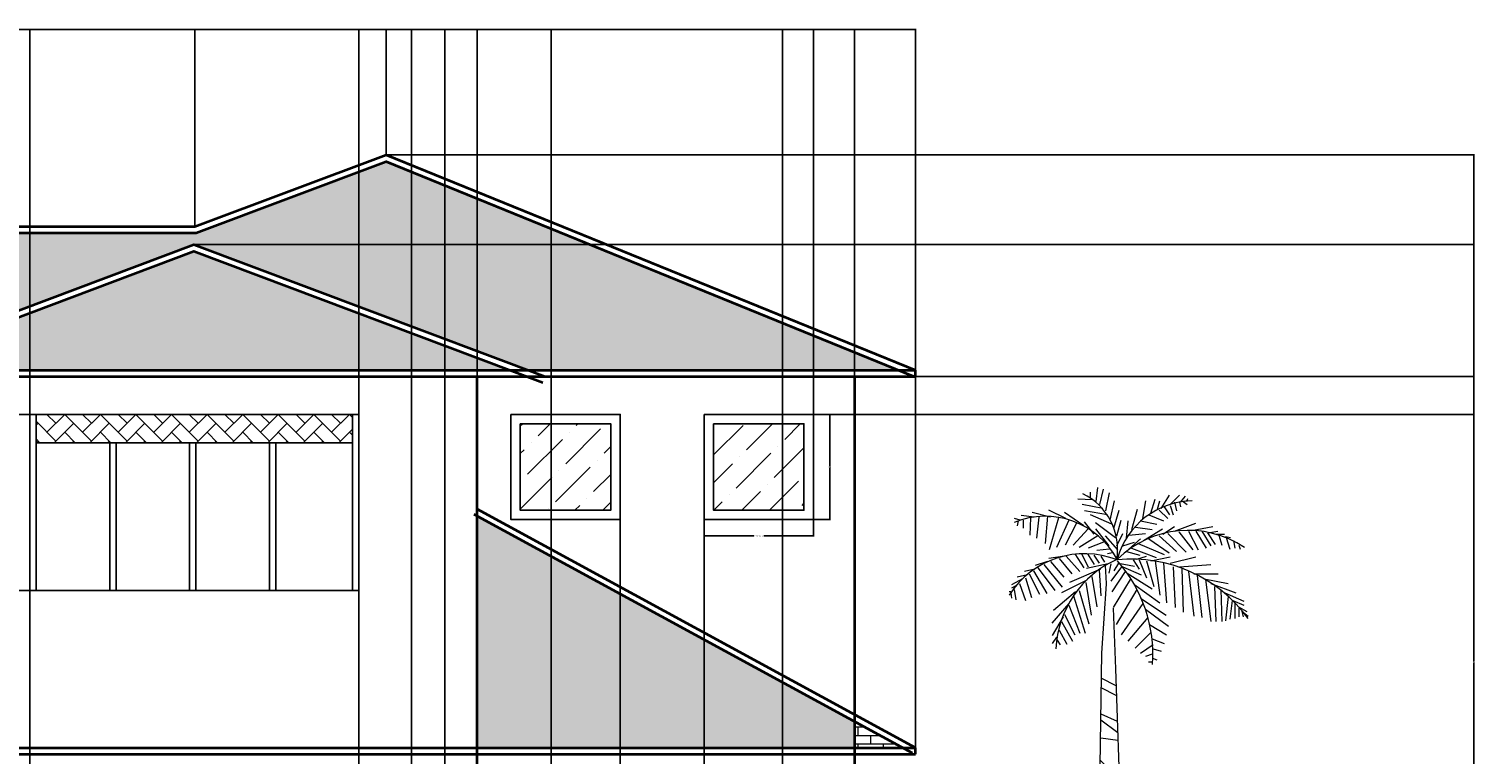
# Model space of a CAD drawing. Units: inches. Extents: x -177 to 697, y -125 to 346.
# Tile 4 of 4: x 237 to 697, y 116 to 346. Entities that reach past the tile are written whole.
import ezdxf

# ---------------------------------------------------------------- set-up
doc = ezdxf.new("R2010")
doc.units = ezdxf.units.IN
doc.header["$MEASUREMENT"] = 0
for name, color, linetype, lineweight in [('A-ANNO-DIMS', 2, 'Continuous', 18), ('A-GLAZ', 4, 'Continuous', 25), ('A-GLAZ-PATT', 252, 'Continuous', 13), ('A-ROOF', 1, 'Continuous', 35), ('A-ROOF-PATT', 252, 'Continuous', 13), ('A-WALL', 7, 'Continuous', 35), ('L-PLNT', 94, 'Continuous', 13)]:
    doc.layers.add(name, color=color, linetype=linetype, lineweight=lineweight)
doc.styles.get("Standard").update_dxf_attribs({"font": 'arial.ttf'})
doc.dimstyles.get("Standard").update_dxf_attribs({"dimtxt": 0.18, "dimasz": 0.18, "dimexe": 0.18, "dimexo": 0.0625, "dimgap": 0.09, "dimtad": 0, "dimtih": 1, "dimtoh": 1, "dimdec": 4, "dimzin": 0, "dimdsep": 46, "dimtxsty": 'Standard', "dimcen": 0.09, "dimadec": 0, "dimazin": 0, "dimtfac": 1, "dimtdec": 4, "dimtofl": 0, "dimtmove": 0, "dimatfit": 3, "dimfxl": 1, "dimtolj": 1, "dimtzin": 0, "dimarcsym": 0})
pattern_1 = [(0, (-118.8082, -115.7344), (0, 2.667), []), (90, (-118.808, -115.7344), (-4, 2.667), [2.667, -2.667])]

# ---------------------------------------------------------------- blocks, each defined once
blk = doc.blocks.new('*U2')
for p, q in [((-7.5, 199.68), (-7.5, 197.946)), ((-5.567, 196.707), (-4.987, 201.167)), ((-4.407, 195.716), (-3.247, 200.672)), ((-2.474, 193.733), (-1.315, 199.433)), ((15.116, 194.477), (17.822, 198.689)), ((18.015, 195.716), (20.914, 198.689)), ((21.301, 196.459), (22.847, 198.441)), ((-20.064, 191.751), (-25.863, 193.238)), ((-15.232, 191.255), (-20.644, 193.981)), ((-9.433, 189.025), (-15.618, 193.238)), ((-6.727, 197.202), (-11.366, 197.45)), ((-3.441, 194.477), (-10.013, 195.716)), ((-1.894, 192.494), (-9.24, 193.733)), ((-1.121, 190.759), (0.232, 196.955)), ((0.038, 188.281), (1.778, 193.981)), ((5.837, 187.786), (7.577, 194.229)), ((9.317, 191.255), (10.283, 196.955)), ((11.829, 192.99), (13.182, 197.45)), ((13.956, 194.229), (14.729, 196.955)), ((14.536, 193.981), (17.242, 191.255)), ((16.082, 194.972), (17.822, 192.494)), ((18.015, 195.468), (18.981, 192.494)), ((19.368, 196.459), (19.948, 193.733)), ((20.914, 196.459), (21.301, 194.972)), ((22.074, 196.707), (23.427, 195.716)), ((23.234, 196.707), (23.62, 197.698)), ((-29.729, 190.759), (-31.469, 191.255)), ((-30.309, 190.512), (-30.695, 189.025)), ((-25.283, 191.751), (-29.342, 192.246)), ((-28.763, 190.759), (-28.763, 188.281)), ((-26.443, 191.503), (-26.636, 186.051)), ((-23.737, 191.751), (-24.51, 185.06)), ((-21.031, 191.998), (-21.804, 183.325)), ((-17.551, 191.503), (-20.451, 181.343)), ((-14.265, 190.759), (-18.131, 182.086)), ((-11.753, 189.768), (-15.425, 182.83)), ((-6.147, 186.299), (-9.24, 190.264)), ((-0.541, 189.52), (-7.307, 192.494)), ((-5.76, 190.016), (0.618, 185.308)), ((1.005, 185.803), (2.358, 190.759)), ((4.098, 185.06), (4.678, 190.512)), ((8.544, 190.512), (13.763, 189.52)), ((11.25, 192.494), (15.889, 190.512)), ((15.695, 186.299), (19.368, 188.777)), ((19.368, 187.29), (26.133, 189.768)), ((24.78, 187.538), (31.546, 188.777)), ((-8.08, 188.034), (-12.912, 182.83)), ((-4.987, 185.803), (-10.979, 182.086)), ((-5.76, 188.034), (-1.508, 182.582)), ((-2.668, 185.803), (1.198, 181.343)), ((1.005, 182.582), (2.938, 186.547)), ((4.871, 186.051), (10.09, 186.547)), ((4.871, 181.591), (8.544, 184.812)), ((6.997, 188.529), (12.216, 187.786)), ((9.51, 184.317), (15.502, 188.034)), ((11.25, 184.812), (17.628, 180.352)), ((14.536, 185.803), (19.948, 180.847)), ((17.242, 186.547), (23.041, 180.599)), ((20.721, 187.042), (25.167, 181.343)), ((23.814, 187.29), (26.907, 181.343)), ((26.133, 187.29), (29.419, 181.838)), ((28.066, 187.29), (30.966, 182.582)), ((29.806, 186.795), (32.319, 183.078)), ((29.999, 186.795), (33.092, 187.29)), ((32.512, 186.299), (35.218, 186.299)), ((33.479, 186.051), (34.445, 182.83)), ((35.605, 185.556), (37.151, 185.308)), ((35.798, 185.308), (36.958, 181.591)), ((38.118, 184.317), (38.504, 181.838)), ((-15.618, 179.36), (-20.644, 178.617)), ((-15.038, 179.36), (-10.786, 174.404)), ((-12.332, 180.104), (-9.433, 175.643)), ((-10.206, 180.104), (-8.08, 175.891)), ((-8.273, 180.104), (-6.147, 176.635)), ((-3.247, 183.821), (-8.08, 181.838)), ((-6.34, 179.608), (-4.6, 177.13)), ((-1.315, 181.591), (-5.374, 181.095)), ((-4.021, 179.36), (-2.861, 177.378)), ((-0.348, 180.352), (-1.894, 180.104)), ((2.938, 182.582), (6.61, 183.821)), ((4.098, 180.847), (8.35, 179.608)), ((5.644, 181.838), (13.569, 178.865)), ((7.384, 178.369), (10.476, 179.36)), ((7.77, 183.325), (16.082, 179.856)), ((39.857, 182.83), (40.244, 181.591)), ((-25.09, 175.148), (-28.376, 174.404)), ((-21.031, 177.626), (-24.897, 176.387)), ((-24.317, 175.891), (-18.711, 168.457)), ((-22.191, 176.635), (-16.391, 169.448)), ((-20.064, 177.626), (-15.812, 172.67)), ((-17.358, 178.617), (-13.299, 173.661)), ((-4.214, 175.148), (-14.072, 170.935)), ((-1.701, 176.882), (-8.66, 175.396)), ((-4.6, 174.9), (-4.021, 166.722)), ((-2.668, 176.387), (-2.376, 170.594)), ((-0.928, 176.882), (-1.508, 173.909)), ((2.551, 175.891), (-0.928, 171.431)), ((1.585, 177.13), (0.038, 174.652)), ((1.585, 177.13), (6.61, 176.139)), ((2.938, 175.891), (8.737, 173.413)), ((6.224, 178.121), (8.157, 175.148)), ((8.157, 178.121), (10.476, 172.422)), ((10.476, 177.874), (12.796, 169.696)), ((11.829, 177.874), (18.015, 179.113)), ((13.182, 177.874), (14.729, 166.97)), ((15.889, 177.13), (16.855, 164.492)), ((18.015, 177.13), (26.133, 179.113)), ((18.981, 175.891), (19.561, 163.005)), ((20.914, 175.891), (30.966, 176.635)), ((21.688, 175.396), (22.074, 161.518)), ((-28.956, 172.174), (-32.435, 170.192)), ((-27.409, 173.413), (-30.695, 172.67)), ((-29.922, 170.687), (-27.989, 165.235)), ((-27.989, 172.422), (-26.056, 166.227)), ((-26.829, 173.661), (-23.544, 167.218)), ((-25.476, 174.652), (-21.224, 167.466)), ((-8.466, 171.678), (-16.585, 167.713)), ((-8.853, 170.935), (-7.113, 160.527)), ((-6.92, 172.917), (-5.374, 163.253)), ((3.711, 174.404), (-0.541, 167.961)), ((5.257, 171.926), (-0.155, 163.005)), ((4.291, 173.909), (12.216, 168.953)), ((6.417, 170.439), (14.729, 164.492)), ((23.814, 174.404), (25.554, 160.279)), ((25.554, 173.661), (33.285, 173.661)), ((26.52, 173.165), (28.066, 159.784)), ((28.839, 172.174), (36.378, 170.687)), ((29.226, 171.926), (30.966, 158.545)), ((30.966, 170.687), (38.891, 167.713)), ((-32.628, 167.961), (-33.208, 167.961)), ((-32.628, 167.713), (-32.435, 165.979)), ((-31.082, 169.944), (-32.435, 169.2)), ((-31.662, 168.705), (-31.082, 165.483)), ((-12.139, 167.961), (-19.098, 162.014)), ((-12.719, 166.722), (-9.046, 154.828)), ((-10.979, 168.457), (-7.887, 157.801)), ((7.384, 168.705), (0.812, 157.553)), ((8.544, 165.979), (16.662, 160.527)), ((32.126, 169.696), (32.512, 158.545)), ((34.058, 168.705), (34.445, 158.545)), ((35.412, 167.713), (41.404, 164.988)), ((36.378, 166.474), (35.605, 158.792)), ((-14.265, 164.244), (-19.678, 158.049)), ((-14.265, 163.749), (-10.786, 154.828)), ((9.317, 164.244), (2.358, 154.332)), ((10.09, 162.51), (17.435, 157.058)), ((37.731, 165.235), (36.958, 159.288)), ((37.924, 165.235), (41.404, 163.749)), ((38.504, 164.492), (38.504, 159.536)), ((39.664, 163.253), (42.37, 161.766)), ((39.857, 162.757), (39.857, 160.031)), ((40.824, 161.766), (41.21, 160.031)), ((41.21, 161.518), (42.757, 160.279)), ((-16.005, 160.031), (-19.484, 154.084)), ((-16.585, 158.545), (-13.106, 152.35)), ((-15.618, 160.775), (-12.332, 154.332)), ((10.863, 159.784), (4.484, 152.35)), ((11.443, 157.553), (16.855, 154.332)), ((-18.131, 153.589), (-19.484, 151.606)), ((-17.938, 152.597), (-16.972, 151.111)), ((-17.358, 155.819), (-14.845, 151.358)), ((11.829, 155.075), (6.804, 150.119)), ((12.216, 153.093), (16.082, 151.606)), ((12.603, 151.111), (8.544, 148.385)), ((12.216, 148.137), (10.09, 147.393)), ((12.603, 149.872), (15.116, 149.128)), ((12.409, 145.659), (11.056, 145.659)), ((12.409, 146.898), (13.763, 146.402)), ((-4.081, 140.645), (0.753, 138.261)), ((-4.081, 137.547), (0.753, 135.163)), ((-4.081, 129.205), (1.124, 126.821)), ((-4.081, 127.298), (1.31, 123.246)), ((-4.081, 121.578), (1.31, 120.863)), ((-4.453, 112.283), (1.682, 105.133)), ((-4.267, 114.428), (1.682, 108.708)), ((-4.639, 102.273), (1.868, 100.604)), ((-4.453, 99.651), (2.24, 98.459)), ((-4.453, 91.071), (2.426, 89.641)), ((-4.825, 83.921), (2.612, 81.061)), ((-4.639, 81.299), (2.797, 78.916)), ((-4.639, 78.916), (2.797, 76.771))]:
    blk.add_line(p, q)
for points in [[(-2.363, 170.553), (-3.88, 148.505), (-4.988, 69.634), (-3.325, 24.869), (0, 0)], [(-0.116, 162.848), (0.554, 143.532), (2.217, 96.635), (3.88, 44.054), (7.76, 12.079), (11.64, 0)]]:
    blk.add_lwpolyline(points)
for centre, radius, start, end in [((-18.427, 181.448), 19.715, 350.285, 64.11229), ((25.595, 171.567), 25.395, 91.40319, 163.882), ((-21.738, 166.094), 25.899, 27.67115, 112.5305), ((23.687, 155.341), 32.188, 56.19272, 134.3213), ((-9.259, 151.732), 28.386, 68.38311, 147.5322), ((14.394, 148.393), 32.752, 113.7592, 177.4133), ((5.828, 132.718), 45.639, 35.98777, 95.82273), ((-32.8, 147.923), 45.309, 356.1943, 41.37848)]:
    blk.add_arc(centre, radius, start, end)
blk = doc.blocks.new('WIN-SINGLE-UPPER-ELEV')
for points in [[(0, 33.46), (34.76, 33.46), (34.76, 0), (0, 0)], [(3, 30.46), (31.76, 30.46), (31.76, 3), (3, 3)]]:
    blk.add_lwpolyline(points, close=True)
blk = doc.blocks.new('*D11')
at = {"layer": 'A-ANNO-DIMS', "color": 0, "lineweight": -2, "transparency": 16777216}
for p, q in [((452.18, 190.16), (452.18, 184.83)), ((486.94, 190.16), (486.94, 184.83)), ((452.36, 185.01), (467.98, 185.01)), ((486.76, 185.01), (471.14, 185.01))]:
    blk.add_line(p, q, dxfattribs=at)
at = {"layer": 'A-ANNO-DIMS', "color": 0, "transparency": 16777216}
for points in [[(452.36, 185.04), (452.36, 184.98), (452.18, 185.01)], [(486.76, 185.04), (486.76, 184.98), (486.94, 185.01)]]:
    blk.add_solid(points, dxfattribs=at)
at = {"layer": 'Defpoints', "color": 0, "transparency": 16777216}
for p in [(452.18, 190.22), (486.94, 190.22), (486.94, 185.01)]:
    blk.add_point(p, dxfattribs=at)
at = {"layer": 'A-ANNO-DIMS', "color": 0, "transparency": 16777216, "insert": (469.56, 185.01), "char_height": 0.18, "attachment_point": 5}
blk.add_mtext('\\A1;UPPER WINDOW 35 TYP.', dxfattribs=at)
blk = doc.blocks.new('*D12')
at = {"layer": 'A-ANNO-DIMS', "color": 0, "lineweight": -2, "transparency": 16777216}
for p, q in [((487, 223.68), (492.33, 223.68)), ((492.15, 223.5), (492.15, 207.13)), ((492.15, 190.4), (492.15, 206.77)), ((487, 190.22), (492.33, 190.22))]:
    blk.add_line(p, q, dxfattribs=at)
at = {"layer": 'A-ANNO-DIMS', "color": 0, "transparency": 16777216}
for points in [[(492.12, 223.5), (492.18, 223.5), (492.15, 223.68)], [(492.12, 190.4), (492.18, 190.4), (492.15, 190.22)]]:
    blk.add_solid(points, dxfattribs=at)
at = {"layer": 'Defpoints', "color": 0, "transparency": 16777216}
for p in [(486.94, 223.68), (492.15, 223.68), (486.94, 190.22)]:
    blk.add_point(p, dxfattribs=at)
at = {"layer": 'A-ANNO-DIMS', "color": 0, "transparency": 16777216, "insert": (492.15, 206.95), "char_height": 0.18, "attachment_point": 5}
blk.add_mtext('\\A1;33 TYP.', dxfattribs=at)
blk = doc.blocks.new('*D20')
at = {"layer": 'A-ANNO-DIMS', "color": 0, "lineweight": -2, "transparency": 16777216}
for p, q in [((351.15, 306.24), (697.14, 306.24)), ((696.96, 306.06), (696.96, 145.14)), ((696.96, -16.14), (696.96, 144.78)), ((500.11, -16.32), (697.14, -16.32))]:
    blk.add_line(p, q, dxfattribs=at)
at = {"layer": 'A-ANNO-DIMS', "color": 0, "transparency": 16777216}
for points in [[(696.93, 306.06), (696.99, 306.06), (696.96, 306.24)], [(696.93, -16.14), (696.99, -16.14), (696.96, -16.32)]]:
    blk.add_solid(points, dxfattribs=at)
at = {"layer": 'Defpoints', "color": 0, "transparency": 16777216}
for p in [(351.08, 306.24), (696.96, 306.24), (500.05, -16.32)]:
    blk.add_point(p, dxfattribs=at)
at = {"layer": 'A-ANNO-DIMS', "color": 0, "transparency": 16777216, "insert": (696.96, 144.96), "char_height": 0.18, "attachment_point": 5}
blk.add_mtext('\\A1;322.56', dxfattribs=at)
blk = doc.blocks.new('*D21')
at = {"layer": 'A-ANNO-DIMS', "color": 0, "lineweight": -2, "transparency": 16777216}
for p, q in [((1.05, 117.74), (1.05, 346.22)), ((1.23, 346.04), (259.84, 346.04)), ((519.23, 346.04), (260.62, 346.04)), ((519.41, 117.74), (519.41, 346.22))]:
    blk.add_line(p, q, dxfattribs=at)
at = {"layer": 'A-ANNO-DIMS', "color": 0, "transparency": 16777216}
for points in [[(1.23, 346.07), (1.23, 346.01), (1.05, 346.04)], [(519.23, 346.07), (519.23, 346.01), (519.41, 346.04)]]:
    blk.add_solid(points, dxfattribs=at)
at = {"layer": 'Defpoints', "color": 0, "transparency": 16777216}
for p in [(519.41, 346.04), (1.05, 117.68), (519.41, 117.68)]:
    blk.add_point(p, dxfattribs=at)
at = {"layer": 'A-ANNO-DIMS', "color": 0, "transparency": 16777216, "insert": (260.23, 346.04), "char_height": 0.18, "attachment_point": 5}
blk.add_mtext('\\A1;518.4', dxfattribs=at)
blk = doc.blocks.new('*D27')
at = {"layer": 'A-ANNO-DIMS', "color": 0, "lineweight": -2, "transparency": 16777216}
for p, q in [((359.12, 19.74), (359.12, 346.22)), ((359.3, 346.04), (363.96, 346.04)), ((369.54, 346.04), (364.87, 346.04)), ((369.72, 19.74), (369.72, 346.22))]:
    blk.add_line(p, q, dxfattribs=at)
at = {"layer": 'A-ANNO-DIMS', "color": 0, "transparency": 16777216}
for points in [[(359.3, 346.07), (359.3, 346.01), (359.12, 346.04)], [(369.54, 346.07), (369.54, 346.01), (369.72, 346.04)]]:
    blk.add_solid(points, dxfattribs=at)
at = {"layer": 'Defpoints', "color": 0, "transparency": 16777216}
for p in [(359.12, 346.04), (359.12, 19.68), (369.72, 19.68)]:
    blk.add_point(p, dxfattribs=at)
at = {"layer": 'A-ANNO-DIMS', "color": 0, "transparency": 16777216, "insert": (364.42, 346.04), "char_height": 0.18, "attachment_point": 5}
blk.add_mtext('\\A1;10.604', dxfattribs=at)
blk = doc.blocks.new('*D29')
at = {"layer": 'A-ANNO-DIMS', "color": 0, "lineweight": -2, "transparency": 16777216}
for p, q in [((200.05, 235.74), (200.05, 346.22)), ((200.23, 346.04), (289.77, 346.04)), ((379.87, 346.04), (290.33, 346.04)), ((380.05, 235.74), (380.05, 346.22))]:
    blk.add_line(p, q, dxfattribs=at)
at = {"layer": 'A-ANNO-DIMS', "color": 0, "transparency": 16777216}
for points in [[(200.23, 346.07), (200.23, 346.01), (200.05, 346.04)], [(379.87, 346.07), (379.87, 346.01), (380.05, 346.04)]]:
    blk.add_solid(points, dxfattribs=at)
at = {"layer": 'Defpoints', "color": 0, "transparency": 16777216}
for p in [(380.05, 346.04), (200.05, 235.68), (380.05, 235.68)]:
    blk.add_point(p, dxfattribs=at)
at = {"layer": 'A-ANNO-DIMS', "color": 0, "transparency": 16777216, "insert": (290.05, 346.04), "char_height": 0.18, "attachment_point": 5}
blk.add_mtext('\\A1;180', dxfattribs=at)
blk = doc.blocks.new('*D32')
at = {"layer": 'A-ANNO-DIMS', "color": 0, "lineweight": -2, "transparency": 16777216}
for p, q in [((237.75, 103.74), (237.75, 346.22)), ((237.93, 346.04), (289.66, 346.04)), ((342.17, 346.04), (290.43, 346.04)), ((342.35, 103.74), (342.35, 346.22))]:
    blk.add_line(p, q, dxfattribs=at)
at = {"layer": 'A-ANNO-DIMS', "color": 0, "transparency": 16777216}
for points in [[(237.93, 346.07), (237.93, 346.01), (237.75, 346.04)], [(342.17, 346.07), (342.17, 346.01), (342.35, 346.04)]]:
    blk.add_solid(points, dxfattribs=at)
at = {"layer": 'Defpoints', "color": 0, "transparency": 16777216}
for p in [(342.35, 346.04), (237.75, 103.68), (342.35, 103.68)]:
    blk.add_point(p, dxfattribs=at)
at = {"layer": 'A-ANNO-DIMS', "color": 0, "transparency": 16777216, "insert": (290.05, 346.04), "char_height": 0.18, "attachment_point": 5}
blk.add_mtext('\\A1;104.6', dxfattribs=at)
blk = doc.blocks.new('*D34')
at = {"layer": 'A-ANNO-DIMS', "color": 0, "lineweight": -2, "transparency": 16777216}
for p, q in [((237.69, 223.68), (-176.98, 223.68)), ((-176.8, 223.5), (-176.8, 195.86)), ((-176.8, 167.85), (-176.8, 195.49)), ((237.69, 167.67), (-176.98, 167.67))]:
    blk.add_line(p, q, dxfattribs=at)
at = {"layer": 'A-ANNO-DIMS', "color": 0, "transparency": 16777216}
for points in [[(-176.83, 223.5), (-176.77, 223.5), (-176.8, 223.68)], [(-176.83, 167.85), (-176.77, 167.85), (-176.8, 167.67)]]:
    blk.add_solid(points, dxfattribs=at)
at = {"layer": 'Defpoints', "color": 0, "transparency": 16777216}
for p in [(-176.8, 223.68), (237.75, 223.68), (237.75, 167.67)]:
    blk.add_point(p, dxfattribs=at)
at = {"layer": 'A-ANNO-DIMS', "color": 0, "transparency": 16777216, "insert": (-176.8, 195.68), "char_height": 0.18, "attachment_point": 5}
blk.add_mtext('\\A1;56.01', dxfattribs=at)
blk = doc.blocks.new('*D35')
at = {"layer": 'A-ANNO-DIMS', "color": 0, "lineweight": -2, "transparency": 16777216}
for p, q in [((380.05, 193.5), (380.05, -124.85)), ((342.35, 167.61), (342.35, -124.85)), ((342.53, -124.67), (360.87, -124.67)), ((379.87, -124.67), (361.52, -124.67))]:
    blk.add_line(p, q, dxfattribs=at)
at = {"layer": 'A-ANNO-DIMS', "color": 0, "transparency": 16777216}
for points in [[(342.53, -124.64), (342.53, -124.7), (342.35, -124.67)], [(379.87, -124.64), (379.87, -124.7), (380.05, -124.67)]]:
    blk.add_solid(points, dxfattribs=at)
at = {"layer": 'Defpoints', "color": 0, "transparency": 16777216}
for p in [(380.05, 193.56), (342.35, 167.67), (380.05, -124.67)]:
    blk.add_point(p, dxfattribs=at)
at = {"layer": 'A-ANNO-DIMS', "color": 0, "transparency": 16777216, "insert": (361.2, -124.67), "char_height": 0.18, "attachment_point": 5}
blk.add_mtext('\\A1;37.7', dxfattribs=at)
blk = doc.blocks.new('*D40')
at = {"layer": 'A-ANNO-DIMS', "color": 0, "lineweight": -2, "transparency": 16777216}
for p, q in [((477.13, 56.7), (477.13, 346.22)), ((477.31, 346.04), (488.2, 346.04)), ((499.87, 346.04), (488.98, 346.04)), ((500.05, 19.74), (500.05, 346.22))]:
    blk.add_line(p, q, dxfattribs=at)
at = {"layer": 'A-ANNO-DIMS', "color": 0, "transparency": 16777216}
for points in [[(477.31, 346.07), (477.31, 346.01), (477.13, 346.04)], [(499.87, 346.07), (499.87, 346.01), (500.05, 346.04)]]:
    blk.add_solid(points, dxfattribs=at)
at = {"layer": 'Defpoints', "color": 0, "transparency": 16777216}
for p in [(477.13, 346.04), (477.13, 56.63), (500.05, 19.68)]:
    blk.add_point(p, dxfattribs=at)
at = {"layer": 'A-ANNO-DIMS', "color": 0, "transparency": 16777216, "insert": (488.59, 346.04), "char_height": 0.18, "attachment_point": 5}
blk.add_mtext('\\A1;22.92', dxfattribs=at)
blk = doc.blocks.new('*D42')
at = {"layer": 'A-ANNO-DIMS', "color": 0, "lineweight": -2, "transparency": 16777216}
for p, q in [((425.51, 190.16), (425.51, -124.85)), ((452.18, 190.16), (452.18, -124.85)), ((425.69, -124.67), (438.45, -124.67)), ((452, -124.67), (439.24, -124.67))]:
    blk.add_line(p, q, dxfattribs=at)
at = {"layer": 'A-ANNO-DIMS', "color": 0, "transparency": 16777216}
for points in [[(425.69, -124.64), (425.69, -124.7), (425.51, -124.67)], [(452, -124.64), (452, -124.7), (452.18, -124.67)]]:
    blk.add_solid(points, dxfattribs=at)
at = {"layer": 'Defpoints', "color": 0, "transparency": 16777216}
for p in [(425.51, 190.22), (452.18, 190.22), (452.18, -124.67)]:
    blk.add_point(p, dxfattribs=at)
at = {"layer": 'A-ANNO-DIMS', "color": 0, "transparency": 16777216, "insert": (438.84, -124.67), "char_height": 0.18, "attachment_point": 5}
blk.add_mtext('\\A1;26.67', dxfattribs=at)
blk = doc.blocks.new('*D44')
at = {"layer": 'A-ANNO-DIMS', "color": 0, "lineweight": -2, "transparency": 16777216}
for p, q in [((486.94, 223.74), (486.94, 346.22)), ((487.12, 346.04), (493.13, 346.04)), ((499.87, 346.04), (493.86, 346.04)), ((500.05, 235.74), (500.05, 346.22))]:
    blk.add_line(p, q, dxfattribs=at)
at = {"layer": 'A-ANNO-DIMS', "color": 0, "transparency": 16777216}
for points in [[(487.12, 346.07), (487.12, 346.01), (486.94, 346.04)], [(499.87, 346.07), (499.87, 346.01), (500.05, 346.04)]]:
    blk.add_solid(points, dxfattribs=at)
at = {"layer": 'Defpoints', "color": 0, "transparency": 16777216}
for p in [(486.94, 346.04), (500.05, 235.68), (486.94, 223.68)]:
    blk.add_point(p, dxfattribs=at)
at = {"layer": 'A-ANNO-DIMS', "color": 0, "transparency": 16777216, "insert": (493.49, 346.04), "char_height": 0.18, "attachment_point": 5}
blk.add_mtext('\\A1;13.11', dxfattribs=at)
blk = doc.blocks.new('*D45')
at = {"layer": 'A-ANNO-DIMS', "color": 0, "lineweight": -2, "transparency": 16777216}
for p, q in [((519.48, 235.68), (697.14, 235.68)), ((696.96, 235.5), (696.96, 229.86)), ((696.96, 223.86), (696.96, 229.5)), ((487, 223.68), (697.14, 223.68))]:
    blk.add_line(p, q, dxfattribs=at)
at = {"layer": 'A-ANNO-DIMS', "color": 0, "transparency": 16777216}
for points in [[(696.93, 235.5), (696.99, 235.5), (696.96, 235.68)], [(696.93, 223.86), (696.99, 223.86), (696.96, 223.68)]]:
    blk.add_solid(points, dxfattribs=at)
at = {"layer": 'Defpoints', "color": 0, "transparency": 16777216}
for p in [(519.41, 235.68), (486.94, 223.68), (696.96, 223.68)]:
    blk.add_point(p, dxfattribs=at)
at = {"layer": 'A-ANNO-DIMS', "color": 0, "transparency": 16777216, "insert": (696.96, 229.68), "char_height": 0.18, "attachment_point": 5}
blk.add_mtext('\\A1;12', dxfattribs=at)
blk = doc.blocks.new('*D47')
at = {"layer": 'A-ANNO-DIMS', "color": 0, "lineweight": -2, "transparency": 16777216}
for p, q in [((160.63, 283.45), (160.63, 346.22)), ((160.81, 346.04), (224.99, 346.04)), ((290.08, 346.04), (225.9, 346.04)), ((290.26, 283.45), (290.26, 346.22))]:
    blk.add_line(p, q, dxfattribs=at)
at = {"layer": 'A-ANNO-DIMS', "color": 0, "transparency": 16777216}
for points in [[(160.81, 346.07), (160.81, 346.01), (160.63, 346.04)], [(290.08, 346.07), (290.08, 346.01), (290.26, 346.04)]]:
    blk.add_solid(points, dxfattribs=at)
at = {"layer": 'Defpoints', "color": 0, "transparency": 16777216}
for p in [(290.26, 346.04), (160.63, 283.39), (290.26, 283.39)]:
    blk.add_point(p, dxfattribs=at)
at = {"layer": 'A-ANNO-DIMS', "color": 0, "transparency": 16777216, "insert": (225.44, 346.04), "char_height": 0.18, "attachment_point": 5}
blk.add_mtext('\\A1;129.63', dxfattribs=at)
blk = doc.blocks.new('*D48')
at = {"layer": 'A-ANNO-DIMS', "color": 0, "lineweight": -2, "transparency": 16777216}
for p, q in [((290.26, 283.45), (290.26, 346.22)), ((290.44, 346.04), (320.28, 346.04)), ((350.9, 346.04), (321.06, 346.04)), ((351.08, 306.3), (351.08, 346.22))]:
    blk.add_line(p, q, dxfattribs=at)
at = {"layer": 'A-ANNO-DIMS', "color": 0, "transparency": 16777216}
for points in [[(290.44, 346.07), (290.44, 346.01), (290.26, 346.04)], [(350.9, 346.07), (350.9, 346.01), (351.08, 346.04)]]:
    blk.add_solid(points, dxfattribs=at)
at = {"layer": 'Defpoints', "color": 0, "transparency": 16777216}
for p in [(351.08, 346.04), (351.08, 306.24), (290.26, 283.39)]:
    blk.add_point(p, dxfattribs=at)
at = {"layer": 'A-ANNO-DIMS', "color": 0, "transparency": 16777216, "insert": (320.67, 346.04), "char_height": 0.18, "attachment_point": 5}
blk.add_mtext('\\A1;60.83', dxfattribs=at)
blk = doc.blocks.new('*D50')
at = {"layer": 'A-ANNO-DIMS', "color": 0, "lineweight": -2, "transparency": 16777216}
for p, q in [((403.53, -16.26), (403.53, 346.22)), ((403.71, 346.04), (451.4, 346.04)), ((499.87, 346.04), (452.18, 346.04)), ((500.05, -16.26), (500.05, 346.22))]:
    blk.add_line(p, q, dxfattribs=at)
at = {"layer": 'A-ANNO-DIMS', "color": 0, "transparency": 16777216}
for points in [[(403.71, 346.07), (403.71, 346.01), (403.53, 346.04)], [(499.87, 346.07), (499.87, 346.01), (500.05, 346.04)]]:
    blk.add_solid(points, dxfattribs=at)
at = {"layer": 'Defpoints', "color": 0, "transparency": 16777216}
for p in [(500.05, 346.04), (403.53, -16.32), (500.05, -16.32)]:
    blk.add_point(p, dxfattribs=at)
at = {"layer": 'A-ANNO-DIMS', "color": 0, "transparency": 16777216, "insert": (451.79, 346.04), "char_height": 0.18, "attachment_point": 5}
blk.add_mtext('\\A1;96.52', dxfattribs=at)
blk = doc.blocks.new('*D53')
at = {"layer": 'A-ANNO-DIMS', "color": 0, "lineweight": -2, "transparency": 16777216}
for p, q in [((351.15, 306.24), (697.14, 306.24)), ((696.96, 306.06), (696.96, 292.14)), ((696.96, 277.86), (696.96, 291.78)), ((290.01, 277.68), (697.14, 277.68))]:
    blk.add_line(p, q, dxfattribs=at)
at = {"layer": 'A-ANNO-DIMS', "color": 0, "transparency": 16777216}
for points in [[(696.93, 306.06), (696.99, 306.06), (696.96, 306.24)], [(696.93, 277.86), (696.99, 277.86), (696.96, 277.68)]]:
    blk.add_solid(points, dxfattribs=at)
at = {"layer": 'Defpoints', "color": 0, "transparency": 16777216}
for p in [(351.08, 306.24), (696.96, 306.24), (289.95, 277.68)]:
    blk.add_point(p, dxfattribs=at)
at = {"layer": 'A-ANNO-DIMS', "color": 0, "transparency": 16777216, "insert": (696.96, 291.96), "char_height": 0.18, "attachment_point": 5}
blk.add_mtext('\\A1;28.56', dxfattribs=at)

msp = doc.modelspace()

# ---------------------------------------------------------------- hatches: boundary and pattern name
at = {"layer": 'A-GLAZ-PATT'}
h = msp.add_hatch(dxfattribs=at)
h.set_pattern_fill('AR-HBONE', color=256)
h.set_pattern_definition([(45, (-118.808, -115.7344), (0, 5.656854), [12, -4]), (135, (-115.9797, -112.906), (4e-16, 5.656854), [12, -4])])
h.paths.add_polyline_path([(340.3468, 223.6802), (239.7524, 223.6802), (239.7524, 214.6802), (340.3468, 214.6802)])
h.paths.add_polyline_path([(340.3468, 103.6802), (239.7524, 103.6802), (239.7524, 94.6802), (340.3468, 94.6802)])
h = msp.add_hatch(dxfattribs=at)
h.set_pattern_fill('ANSI36', color=256, scale=50)
h.set_pattern_definition([(45, (-118.808, -115.7344), (3.314563, 12.1534), [15.625, -3.125, 0, -3.125])])
h.paths.add_polyline_path([(422.5056, 220.6802), (393.7433, 220.6802), (393.7433, 193.2226), (422.5056, 193.2226)])
h.paths.add_polyline_path([(483.9391, 220.6802), (455.1768, 220.6802), (455.1768, 193.2226), (483.9391, 193.2226)])
at = {"layer": 'A-ROOF-PATT'}
h = msp.add_hatch(dxfattribs=at)
h.set_pattern_fill('AR-BRSTD', color=256)
h.set_pattern_definition(pattern_1)
h.paths.add_polyline_path([(289.952, 277.6802), (396.2807, 237.6802), (500.0496, 237.6802), (514.1115, 237.6802), (351.0539, 304.0916), (290.6192, 281.3896), (161.1548, 281.3896), (83.9154, 237.6802), (183.6234, 237.6802)])
h.paths.add_polyline_path([(289.952, 275.5434), (189.3036, 237.6802), (390.6005, 237.6802)], flags=17)
h.paths.add_polyline_path([(200.0496, 196.199), (61.0496, 117.6802), (200.0496, 117.6802)])
h.paths.add_polyline_path([(88.5518, 161.6802), (5.3286, 117.6802), (61.0496, 117.6802), (138.9418, 161.6802)])
h.paths.add_polyline_path([(380.0496, 191.2819), (380.0496, 117.6802), (500.0496, 117.6802), (500.0496, 125.9461)])
h = msp.add_hatch(dxfattribs=at)
h.set_pattern_fill('AR-BRSTD', color=256)
h.set_pattern_definition(pattern_1)
h.paths.add_polyline_path([(500.0496, 125.9461), (500.0496, 117.6802), (515.2312, 117.6802)])

# ---------------------------------------------------------------- linework, layer by layer
at = {"layer": 'A-GLAZ'}
for p, q in [((342.3468, 223.6802), (237.7524, 223.6802)), ((237.7524, 223.6802), (237.7524, 167.6715)), ((239.7524, 223.6802), (239.7524, 167.6715)), ((340.3468, 167.6715), (340.3468, 223.6802)), ((342.3468, 167.6715), (342.3468, 223.6802)), ((340.3468, 214.6802), (239.7524, 214.6802)), ((263.1757, 214.6802), (263.1757, 167.6715)), ((265.1757, 214.6802), (265.1757, 167.6715)), ((288.5989, 214.6802), (288.5989, 167.6715)), ((290.5989, 214.6802), (290.5989, 167.6715)), ((314.0222, 214.6802), (314.0222, 167.6715)), ((316.0222, 214.6802), (316.0222, 167.6715)), ((237.7524, 167.6715), (342.3468, 167.6715))]:
    msp.add_line(p, q, dxfattribs=at)
at = {"layer": 'A-ROOF'}
for p, q in [((79.8545, 237.6802), (500.0496, 237.6802)), ((79.8545, 235.6802), (500.0496, 235.6802)), ((500.0496, 237.6802), (519.4137, 237.6802)), ((500.0496, 235.6802), (519.4137, 235.6802)), ((519.4137, 235.6802), (519.4137, 237.6802)), ((519.4137, 237.6802), (519.4137, 237.6802)), ((519.4137, 117.6802), (380.0496, 193.5592)), ((518.4573, 115.9237), (379.0932, 191.8026)), ((1.0496, 117.6802), (500.0496, 117.6802)), ((20.0496, 115.6802), (500.0496, 115.6802)), ((500.0496, 117.6802), (519.4137, 117.6802)), ((500.0496, 115.6802), (519.4137, 115.6802)), ((519.4137, 115.6802), (519.4137, 117.6802))]:
    msp.add_line(p, q, dxfattribs=at)
for points in [[(79.8545, 237.6802), (160.6282, 283.3896), (290.2559, 283.3896), (351.0833, 306.2391), (519.4137, 237.6802)], [(80.8395, 235.9396), (161.1548, 281.3896), (290.6192, 281.3896), (351.0539, 304.0916), (518.6593, 235.828)], [(178.307, 235.6802), (289.952, 277.6802), (401.5971, 235.6802)], [(179.0112, 233.8083), (289.952, 275.5434), (400.8929, 233.8083)]]:
    msp.add_lwpolyline(points, dxfattribs=at)
at = {"layer": 'A-WALL'}
for p, q in [((380.0496, 19.6802), (380.0496, 235.6802)), ((500.0496, 235.6802), (500.0496, -16.3198))]:
    msp.add_line(p, q, dxfattribs=at)

# ---------------------------------------------------------------- block references
at = {"layer": 'A-GLAZ'}
for p in [(390.7433, 190.2226), (452.1768, 190.2226)]:
    msp.add_blockref('WIN-SINGLE-UPPER-ELEV', p, dxfattribs=at)
at = {"layer": 'L-PLNT'}
msp.add_blockref('*U2', (582.3957, -0.7305), dxfattribs=at)

# ---------------------------------------------------------------- dimensions: what is measured, and where the dimension line sits
at = {"layer": 'A-ANNO-DIMS'}
for base, p1, p2, override, picture, middle in [((519.4137, 346.0391), (1.0496, 117.6802), (519.4137, 117.6802), {"dimdec": 1, "dimlfac": 1, "dimrnd": 0, "dimzin": 0, "dimdsep": 46, "dimlunit": 2}, '*D21', (260.2316, 346.0391)), ((290.2559, 346.0391), (160.6282, 283.3896), (290.2559, 283.3896), {"dimdec": 2, "dimlfac": 1, "dimrnd": 0, "dimzin": 0, "dimdsep": 46, "dimlunit": 2}, '*D47', (225.442, 346.0391)), ((380.0496, 346.0391), (200.0496, 235.6802), (380.0496, 235.6802), {"dimdec": 0, "dimlfac": 1, "dimrnd": 0, "dimzin": 0, "dimdsep": 46, "dimlunit": 2}, '*D29', (290.0496, 346.0391)), ((342.3468, 346.0391), (237.7524, 103.6802), (342.3468, 103.6802), {"dimdec": 1, "dimlfac": 1, "dimrnd": 0, "dimzin": 0, "dimdsep": 46, "dimlunit": 2}, '*D32', (290.0496, 346.0391)), ((351.0833, 346.0391), (290.2559, 283.3896), (351.0833, 306.2391), {"dimdec": 2, "dimlfac": 1, "dimrnd": 0, "dimzin": 0, "dimdsep": 46, "dimlunit": 2}, '*D48', (320.6696, 346.0391)), ((359.116, 346.0391), (369.7204, 19.6802), (359.116, 19.6802), {"dimdec": 3, "dimlfac": 1, "dimrnd": 0, "dimzin": 0, "dimdsep": 46, "dimlunit": 2}, '*D27', (364.4182, 346.0391)), ((500.0496, 346.0391), (403.5337, -16.3198), (500.0496, -16.3198), {"dimdec": 2, "dimlfac": 1, "dimrnd": 0, "dimzin": 0, "dimdsep": 46, "dimlunit": 2}, '*D50', (451.7916, 346.0391)), ((477.1317, 346.0391), (500.0496, 19.6802), (477.1317, 56.6343), {"dimdec": 2, "dimlfac": 1, "dimrnd": 0, "dimzin": 0, "dimdsep": 46, "dimlunit": 2}, '*D40', (488.5906, 346.0391)), ((486.9391, 346.0391), (500.0496, 235.6802), (486.9391, 223.6802), {"dimdec": 2, "dimlfac": 1, "dimrnd": 0, "dimzin": 0, "dimdsep": 46, "dimlunit": 2}, '*D44', (493.4943, 346.0391)), ((380.0496, -124.671), (342.3468, 167.6715), (380.0496, 193.5592), {"dimdec": 1, "dimlfac": 1, "dimrnd": 0, "dimzin": 0, "dimdsep": 46, "dimlunit": 2}, '*D35', (361.1982, -124.671)), ((452.1768, -124.671), (425.5056, 190.2226), (452.1768, 190.2226), {"dimdec": 2, "dimlfac": 1, "dimrnd": 0, "dimzin": 0, "dimdsep": 46, "dimlunit": 2}, '*D42', (438.8412, -124.671))]:
    dim = msp.add_linear_dim(base=base, p1=p1, p2=p2, dimstyle='Standard', override=override, dxfattribs=at)
    dim.commit()
    dim.dimension.update_dxf_attribs({"geometry": picture, "text_midpoint": middle})
for base, p1, p2, override, picture, middle in [((696.9617, 306.2391), (289.952, 277.6802), (351.0833, 306.2391), {"dimdec": 2, "dimlfac": 1, "dimrnd": 0, "dimzin": 0, "dimdsep": 46, "dimlunit": 2}, '*D53', (696.9617, 291.9597)), ((696.9617, 306.2391), (500.0496, -16.3198), (351.0833, 306.2391), {"dimdec": 2, "dimlfac": 1, "dimrnd": 0, "dimzin": 0, "dimdsep": 46, "dimlunit": 2}, '*D20', (696.9617, 144.9597)), ((696.9617, 223.6802), (519.4137, 235.6802), (486.9391, 223.6802), {"dimdec": 0, "dimlfac": 1, "dimrnd": 0, "dimzin": 0, "dimdsep": 46, "dimlunit": 2}, '*D45', (696.9617, 229.6802)), ((-176.8039, 223.6802), (237.7524, 167.6715), (237.7524, 223.6802), {"dimdec": 2, "dimlfac": 1, "dimrnd": 0, "dimzin": 0, "dimdsep": 46, "dimlunit": 2}, '*D34', (-176.8039, 195.6759))]:
    dim = msp.add_linear_dim(base=base, p1=p1, p2=p2, angle=90, dimstyle='Standard', override=override, dxfattribs=at)
    dim.commit()
    dim.dimension.update_dxf_attribs({"geometry": picture, "text_midpoint": middle})
dim = msp.add_linear_dim(base=(492.1534, 223.6802), p1=(486.9391, 190.2226), p2=(486.9391, 223.6802), angle=90, text='<> TYP.', dimstyle='Standard', override={"dimdec": 0, "dimlfac": 1, "dimrnd": 0, "dimzin": 0, "dimdsep": 46, "dimlunit": 2}, dxfattribs=at)
dim.commit()
dim.dimension.update_dxf_attribs({"geometry": '*D12', "text_midpoint": (492.1534, 206.9514)})
dim = msp.add_linear_dim(base=(486.9391, 185.0083), p1=(452.1768, 190.2226), p2=(486.9391, 190.2226), text='UPPER WINDOW <> TYP.', dimstyle='Standard', override={"dimdec": 0, "dimlfac": 1, "dimrnd": 0, "dimzin": 0, "dimdsep": 46, "dimlunit": 2}, dxfattribs=at)
dim.commit()
dim.dimension.update_dxf_attribs({"geometry": '*D11', "text_midpoint": (469.5579, 185.0083)})

doc.saveas('drawing.dxf')
